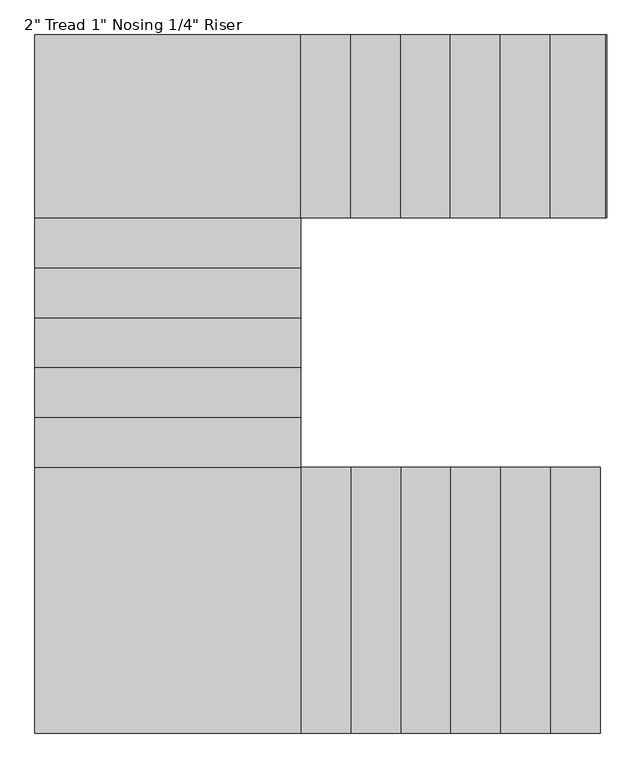
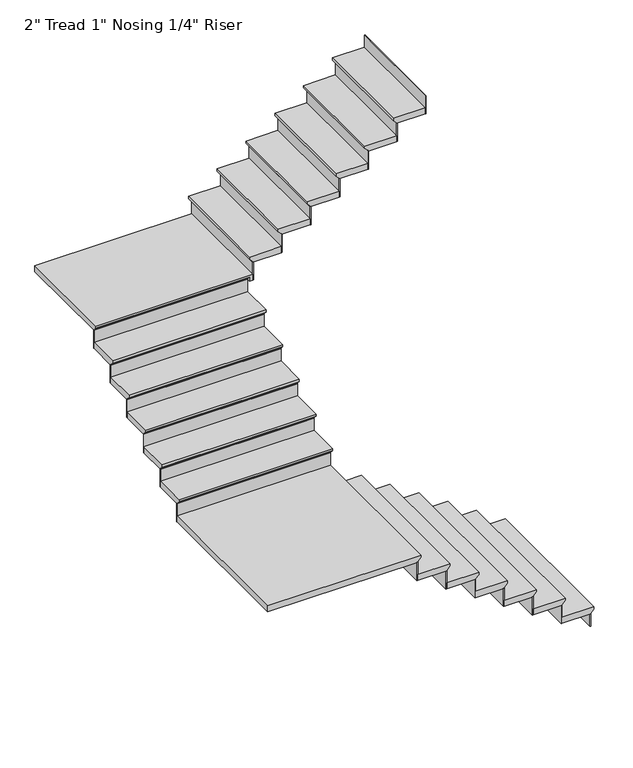
"""IFC4 building model written with IfcOpenShell, lengths in millimetres: stair flight geometry."""

from ifc_helpers import new_model, si_unit, origin, place, context, project, spatial, faceted_brep, source, transform, mapped, element, save


def stair_flight_6293cd8f(model_context):
    return source(origin(), model_context, "Body", "Brep", [
        faceted_brep([(-2515.2117403, -5163.0426559, 133.35), (-2515.2117403, -5163.0426559, 152.4), (-2515.2117403, -6382.2426559, 152.4), (-2515.2117403, -6382.2426559, 133.35), (-2540.6117403, -5163.0426559, 107.95), (-2540.6117403, -6382.2426559, 107.95), (-2769.2117403, -5163.0426559, 152.4), (-2769.2117403, -6382.2426559, 152.4), (-2540.6117403, -6382.2426559, 101.6), (-2769.2117403, -6382.2426559, 101.6), (-2769.2117403, -5163.0426559, 101.6), (-2540.6117403, -5163.0426559, 101.6)], [[[0, 1, 2, 3]], [[4, 0, 3, 5]], [[2, 1, 6, 7]], [[8, 9, 10, 11]], [[2, 7, 9, 8, 5, 3]], [[8, 11, 4, 5]], [[6, 1, 0, 4, 11, 10]], [[7, 6, 10, 9]]]),
        faceted_brep([(-2540.6117403, -5163.0426559, 101.6), (-2540.6117403, -5163.0426559, 0.0), (-2546.9617403, -5163.0426559, 0.0), (-2546.9617403, -5163.0426559, 101.6), (-2540.6117403, -6382.2426559, 101.6), (-2546.9617403, -6382.2426559, 101.6), (-2546.9617403, -6382.2426559, 0.0), (-2540.6117403, -6382.2426559, 0.0)], [[[0, 1, 2, 3]], [[4, 5, 6, 7]], [[1, 0, 4, 7]], [[2, 1, 7, 6]], [[3, 2, 6, 5]], [[0, 3, 5, 4]]]),
        faceted_brep([(-2769.2117403, -5163.0426559, 254.0), (-2769.2117403, -5163.0426559, 101.6), (-2775.5617403, -5163.0426559, 101.6), (-2775.5617403, -5163.0426559, 254.0), (-2769.2117403, -6382.2426559, 254.0), (-2775.5617403, -6382.2426559, 254.0), (-2775.5617403, -6382.2426559, 101.6), (-2769.2117403, -6382.2426559, 101.6)], [[[0, 1, 2, 3]], [[4, 5, 6, 7]], [[1, 0, 4, 7]], [[2, 1, 7, 6]], [[3, 2, 6, 5]], [[0, 3, 5, 4]]]),
        faceted_brep([(-2743.8117403, -6382.2426559, 304.8), (-2743.8117403, -5163.0426559, 304.8), (-2997.8117403, -5163.0426559, 304.8), (-2997.8117403, -6382.2426559, 304.8), (-2769.2117403, -6382.2426559, 254.0), (-2997.8117403, -6382.2426559, 254.0), (-2997.8117403, -5163.0426559, 254.0), (-2769.2117403, -5163.0426559, 254.0), (-2769.2117403, -6382.2426559, 260.35), (-2743.8117403, -6382.2426559, 285.75), (-2769.2117403, -5163.0426559, 260.35), (-2743.8117403, -5163.0426559, 285.75)], [[[0, 1, 2, 3]], [[4, 5, 6, 7]], [[0, 3, 5, 4, 8, 9]], [[4, 7, 10, 8]], [[2, 1, 11, 10, 7, 6]], [[3, 2, 6, 5]], [[11, 1, 0, 9]], [[10, 11, 9, 8]]]),
        faceted_brep([(-2997.8117403, -5163.0426559, 406.4), (-2997.8117403, -5163.0426559, 254.0), (-3004.1617403, -5163.0426559, 254.0), (-3004.1617403, -5163.0426559, 406.4), (-2997.8117403, -6382.2426559, 406.4), (-3004.1617403, -6382.2426559, 406.4), (-3004.1617403, -6382.2426559, 254.0), (-2997.8117403, -6382.2426559, 254.0)], [[[0, 1, 2, 3]], [[4, 5, 6, 7]], [[1, 0, 4, 7]], [[2, 1, 7, 6]], [[3, 2, 6, 5]], [[0, 3, 5, 4]]]),
        faceted_brep([(-2972.4117403, -6382.2426559, 457.2), (-2972.4117403, -5163.0426559, 457.2), (-3226.4117403, -5163.0426559, 457.2), (-3226.4117403, -6382.2426559, 457.2), (-2997.8117403, -6382.2426559, 406.4), (-3226.4117403, -6382.2426559, 406.4), (-3226.4117403, -5163.0426559, 406.4), (-2997.8117403, -5163.0426559, 406.4), (-2997.8117403, -6382.2426559, 412.75), (-2972.4117403, -6382.2426559, 438.15), (-2997.8117403, -5163.0426559, 412.75), (-2972.4117403, -5163.0426559, 438.15)], [[[0, 1, 2, 3]], [[4, 5, 6, 7]], [[0, 3, 5, 4, 8, 9]], [[4, 7, 10, 8]], [[2, 1, 11, 10, 7, 6]], [[3, 2, 6, 5]], [[11, 1, 0, 9]], [[10, 11, 9, 8]]]),
        faceted_brep([(-3226.4117403, -5163.0426559, 558.8), (-3226.4117403, -5163.0426559, 406.4), (-3232.7617403, -5163.0426559, 406.4), (-3232.7617403, -5163.0426559, 558.8), (-3226.4117403, -6382.2426559, 558.8), (-3232.7617403, -6382.2426559, 558.8), (-3232.7617403, -6382.2426559, 406.4), (-3226.4117403, -6382.2426559, 406.4)], [[[0, 1, 2, 3]], [[4, 5, 6, 7]], [[1, 0, 4, 7]], [[2, 1, 7, 6]], [[3, 2, 6, 5]], [[0, 3, 5, 4]]]),
        faceted_brep([(-3201.0117403, -6382.2426559, 609.6), (-3201.0117403, -5163.0426559, 609.6), (-3455.0117403, -5163.0426559, 609.6), (-3455.0117403, -6382.2426559, 609.6), (-3226.4117403, -6382.2426559, 558.8), (-3455.0117403, -6382.2426559, 558.8), (-3455.0117403, -5163.0426559, 558.8), (-3226.4117403, -5163.0426559, 558.8), (-3226.4117403, -6382.2426559, 565.15), (-3201.0117403, -6382.2426559, 590.55), (-3226.4117403, -5163.0426559, 565.15), (-3201.0117403, -5163.0426559, 590.55)], [[[0, 1, 2, 3]], [[4, 5, 6, 7]], [[0, 3, 5, 4, 8, 9]], [[4, 7, 10, 8]], [[2, 1, 11, 10, 7, 6]], [[3, 2, 6, 5]], [[11, 1, 0, 9]], [[10, 11, 9, 8]]]),
        faceted_brep([(-3455.0117403, -5163.0426559, 711.2), (-3455.0117403, -5163.0426559, 558.8), (-3461.3617403, -5163.0426559, 558.8), (-3461.3617403, -5163.0426559, 711.2), (-3455.0117403, -6382.2426559, 711.2), (-3461.3617403, -6382.2426559, 711.2), (-3461.3617403, -6382.2426559, 558.8), (-3455.0117403, -6382.2426559, 558.8)], [[[0, 1, 2, 3]], [[4, 5, 6, 7]], [[1, 0, 4, 7]], [[2, 1, 7, 6]], [[3, 2, 6, 5]], [[0, 3, 5, 4]]]),
        faceted_brep([(-3429.6117403, -6382.2426559, 762.0), (-3429.6117403, -5163.0426559, 762.0), (-3683.6117403, -5163.0426559, 762.0), (-3683.6117403, -6382.2426559, 762.0), (-3455.0117403, -6382.2426559, 711.2), (-3683.6117403, -6382.2426559, 711.2), (-3683.6117403, -5163.0426559, 711.2), (-3455.0117403, -5163.0426559, 711.2), (-3455.0117403, -6382.2426559, 717.55), (-3429.6117403, -6382.2426559, 742.95), (-3455.0117403, -5163.0426559, 717.55), (-3429.6117403, -5163.0426559, 742.95)], [[[0, 1, 2, 3]], [[4, 5, 6, 7]], [[0, 3, 5, 4, 8, 9]], [[4, 7, 10, 8]], [[2, 1, 11, 10, 7, 6]], [[3, 2, 6, 5]], [[11, 1, 0, 9]], [[10, 11, 9, 8]]]),
        faceted_brep([(-3683.6117403, -5163.0426559, 863.6), (-3683.6117403, -5163.0426559, 711.2), (-3689.9617403, -5163.0426559, 711.2), (-3689.9617403, -5163.0426559, 863.6), (-3683.6117403, -6382.2426559, 863.6), (-3689.9617403, -6382.2426559, 863.6), (-3689.9617403, -6382.2426559, 711.2), (-3683.6117403, -6382.2426559, 711.2)], [[[0, 1, 2, 3]], [[4, 5, 6, 7]], [[1, 0, 4, 7]], [[2, 1, 7, 6]], [[3, 2, 6, 5]], [[0, 3, 5, 4]]]),
        faceted_brep([(-3658.2117403, -6382.2426559, 914.4), (-3658.2117403, -5163.0426559, 914.4), (-3912.2117403, -5163.0426559, 914.4), (-3912.2117403, -6382.2426559, 914.4), (-3683.6117403, -6382.2426559, 863.6), (-3912.2117403, -6382.2426559, 863.6), (-3912.2117403, -5163.0426559, 863.6), (-3683.6117403, -5163.0426559, 863.6), (-3683.6117403, -6382.2426559, 869.95), (-3658.2117403, -6382.2426559, 895.35), (-3683.6117403, -5163.0426559, 869.95), (-3658.2117403, -5163.0426559, 895.35)], [[[0, 1, 2, 3]], [[4, 5, 6, 7]], [[0, 3, 5, 4, 8, 9]], [[4, 7, 10, 8]], [[2, 1, 11, 10, 7, 6]], [[3, 2, 6, 5]], [[11, 1, 0, 9]], [[10, 11, 9, 8]]]),
        faceted_brep([(-3912.2117403, -5163.0426559, 1016.0), (-3912.2117403, -5163.0426559, 863.6), (-3918.5617403, -5163.0426559, 863.6), (-3918.5617403, -5163.0426559, 1016.0), (-3912.2117403, -6382.2426559, 1016.0), (-3918.5617403, -6382.2426559, 1016.0), (-3918.5617403, -6382.2426559, 863.6), (-3912.2117403, -6382.2426559, 863.6)], [[[0, 1, 2, 3]], [[4, 5, 6, 7]], [[1, 0, 4, 7]], [[2, 1, 7, 6]], [[3, 2, 6, 5]], [[0, 3, 5, 4]]]),
        faceted_brep([(-5106.0117403, -5137.6426559, 1066.8), (-5106.0117403, -6382.2426559, 1066.8), (-3886.8117403, -6382.2426559, 1066.8), (-3886.8117403, -5137.6426559, 1066.8), (-5106.0117403, -6382.2426559, 1016.0), (-5106.0117403, -5137.6426559, 1016.0), (-3886.8117403, -5137.6426559, 1016.0), (-3886.8117403, -5163.0426559, 1016.0), (-3912.2117403, -5163.0426559, 1016.0), (-3912.2117403, -6382.2426559, 1016.0), (-3912.2117403, -6382.2426559, 1022.35), (-3886.8117403, -6382.2426559, 1047.75), (-3912.2117403, -5163.0426559, 1022.35), (-3886.8117403, -5163.0426559, 1047.75)], [[[0, 1, 2, 3]], [[4, 5, 6, 7, 8, 9]], [[1, 0, 5, 4]], [[2, 1, 4, 9, 10, 11]], [[9, 8, 12, 10]], [[8, 7, 13, 12]], [[3, 2, 11, 13, 7, 6]], [[0, 3, 6, 5]], [[11, 10, 12, 13]]]),
        faceted_brep([(-3886.8117403, -5137.6426559, 1168.4), (-3886.8117403, -5137.6426559, 1016.0), (-3886.8117403, -5131.2926559, 1016.0), (-3886.8117403, -5131.2926559, 1168.4), (-5106.0117403, -5137.6426559, 1168.4), (-5106.0117403, -5131.2926559, 1168.4), (-5106.0117403, -5131.2926559, 1016.0), (-5106.0117403, -5137.6426559, 1016.0)], [[[0, 1, 2, 3]], [[4, 5, 6, 7]], [[1, 0, 4, 7]], [[2, 1, 7, 6]], [[3, 2, 6, 5]], [[0, 3, 5, 4]]]),
        faceted_brep([(-5106.0117403, -5163.0426559, 1219.2), (-3886.8117403, -5163.0426559, 1219.2), (-3886.8117403, -4909.0426559, 1219.2), (-5106.0117403, -4909.0426559, 1219.2), (-5106.0117403, -5137.6426559, 1168.4), (-5106.0117403, -4909.0426559, 1168.4), (-3886.8117403, -4909.0426559, 1168.4), (-3886.8117403, -5137.6426559, 1168.4), (-5106.0117403, -5137.6426559, 1174.75), (-5106.0117403, -5163.0426559, 1200.15), (-3886.8117403, -5137.6426559, 1174.75), (-3886.8117403, -5163.0426559, 1200.15)], [[[0, 1, 2, 3]], [[4, 5, 6, 7]], [[0, 3, 5, 4, 8, 9]], [[4, 7, 10, 8]], [[2, 1, 11, 10, 7, 6]], [[3, 2, 6, 5]], [[11, 1, 0, 9]], [[10, 11, 9, 8]]]),
        faceted_brep([(-3886.8117403, -4909.0426559, 1320.8), (-3886.8117403, -4909.0426559, 1168.4), (-3886.8117403, -4902.6926559, 1168.4), (-3886.8117403, -4902.6926559, 1320.8), (-5106.0117403, -4909.0426559, 1320.8), (-5106.0117403, -4902.6926559, 1320.8), (-5106.0117403, -4902.6926559, 1168.4), (-5106.0117403, -4909.0426559, 1168.4)], [[[0, 1, 2, 3]], [[4, 5, 6, 7]], [[1, 0, 4, 7]], [[2, 1, 7, 6]], [[3, 2, 6, 5]], [[0, 3, 5, 4]]]),
        faceted_brep([(-5106.0117403, -4934.4426559, 1371.6), (-3886.8117403, -4934.4426559, 1371.6), (-3886.8117403, -4680.4426559, 1371.6), (-5106.0117403, -4680.4426559, 1371.6), (-5106.0117403, -4909.0426559, 1320.8), (-5106.0117403, -4680.4426559, 1320.8), (-3886.8117403, -4680.4426559, 1320.8), (-3886.8117403, -4909.0426559, 1320.8), (-5106.0117403, -4909.0426559, 1327.15), (-5106.0117403, -4934.4426559, 1352.55), (-3886.8117403, -4909.0426559, 1327.15), (-3886.8117403, -4934.4426559, 1352.55)], [[[0, 1, 2, 3]], [[4, 5, 6, 7]], [[0, 3, 5, 4, 8, 9]], [[4, 7, 10, 8]], [[2, 1, 11, 10, 7, 6]], [[3, 2, 6, 5]], [[11, 1, 0, 9]], [[10, 11, 9, 8]]]),
        faceted_brep([(-3886.8117403, -4680.4426559, 1473.2), (-3886.8117403, -4680.4426559, 1320.8), (-3886.8117403, -4674.0926559, 1320.8), (-3886.8117403, -4674.0926559, 1473.2), (-5106.0117403, -4680.4426559, 1473.2), (-5106.0117403, -4674.0926559, 1473.2), (-5106.0117403, -4674.0926559, 1320.8), (-5106.0117403, -4680.4426559, 1320.8)], [[[0, 1, 2, 3]], [[4, 5, 6, 7]], [[1, 0, 4, 7]], [[2, 1, 7, 6]], [[3, 2, 6, 5]], [[0, 3, 5, 4]]]),
        faceted_brep([(-5106.0117403, -4705.8426559, 1524.0), (-3886.8117403, -4705.8426559, 1524.0), (-3886.8117403, -4451.8426559, 1524.0), (-5106.0117403, -4451.8426559, 1524.0), (-5106.0117403, -4680.4426559, 1473.2), (-5106.0117403, -4451.8426559, 1473.2), (-3886.8117403, -4451.8426559, 1473.2), (-3886.8117403, -4680.4426559, 1473.2), (-5106.0117403, -4680.4426559, 1479.55), (-5106.0117403, -4705.8426559, 1504.95), (-3886.8117403, -4680.4426559, 1479.55), (-3886.8117403, -4705.8426559, 1504.95)], [[[0, 1, 2, 3]], [[4, 5, 6, 7]], [[0, 3, 5, 4, 8, 9]], [[4, 7, 10, 8]], [[2, 1, 11, 10, 7, 6]], [[3, 2, 6, 5]], [[11, 1, 0, 9]], [[10, 11, 9, 8]]]),
        faceted_brep([(-3886.8117403, -4451.8426559, 1625.6), (-3886.8117403, -4451.8426559, 1473.2), (-3886.8117403, -4445.4926559, 1473.2), (-3886.8117403, -4445.4926559, 1625.6), (-5106.0117403, -4451.8426559, 1625.6), (-5106.0117403, -4445.4926559, 1625.6), (-5106.0117403, -4445.4926559, 1473.2), (-5106.0117403, -4451.8426559, 1473.2)], [[[0, 1, 2, 3]], [[4, 5, 6, 7]], [[1, 0, 4, 7]], [[2, 1, 7, 6]], [[3, 2, 6, 5]], [[0, 3, 5, 4]]]),
        faceted_brep([(-5106.0117403, -4477.2426559, 1676.4), (-3886.8117403, -4477.2426559, 1676.4), (-3886.8117403, -4223.2426559, 1676.4), (-5106.0117403, -4223.2426559, 1676.4), (-5106.0117403, -4451.8426559, 1625.6), (-5106.0117403, -4223.2426559, 1625.6), (-3886.8117403, -4223.2426559, 1625.6), (-3886.8117403, -4451.8426559, 1625.6), (-5106.0117403, -4451.8426559, 1631.95), (-5106.0117403, -4477.2426559, 1657.35), (-3886.8117403, -4451.8426559, 1631.95), (-3886.8117403, -4477.2426559, 1657.35)], [[[0, 1, 2, 3]], [[4, 5, 6, 7]], [[0, 3, 5, 4, 8, 9]], [[4, 7, 10, 8]], [[2, 1, 11, 10, 7, 6]], [[3, 2, 6, 5]], [[11, 1, 0, 9]], [[10, 11, 9, 8]]]),
        faceted_brep([(-3886.8117403, -4223.2426559, 1778.0), (-3886.8117403, -4223.2426559, 1625.6), (-3886.8117403, -4216.8926559, 1625.6), (-3886.8117403, -4216.8926559, 1778.0), (-5106.0117403, -4223.2426559, 1778.0), (-5106.0117403, -4216.8926559, 1778.0), (-5106.0117403, -4216.8926559, 1625.6), (-5106.0117403, -4223.2426559, 1625.6)], [[[0, 1, 2, 3]], [[4, 5, 6, 7]], [[1, 0, 4, 7]], [[2, 1, 7, 6]], [[3, 2, 6, 5]], [[0, 3, 5, 4]]]),
        faceted_brep([(-5106.0117403, -4248.6426559, 1828.8), (-3886.8117403, -4248.6426559, 1828.8), (-3886.8117403, -3994.6426559, 1828.8), (-5106.0117403, -3994.6426559, 1828.8), (-5106.0117403, -4223.2426559, 1778.0), (-5106.0117403, -3994.6426559, 1778.0), (-3886.8117403, -3994.6426559, 1778.0), (-3886.8117403, -4223.2426559, 1778.0), (-5106.0117403, -4223.2426559, 1784.35), (-5106.0117403, -4248.6426559, 1809.75), (-3886.8117403, -4223.2426559, 1784.35), (-3886.8117403, -4248.6426559, 1809.75)], [[[0, 1, 2, 3]], [[4, 5, 6, 7]], [[0, 3, 5, 4, 8, 9]], [[4, 7, 10, 8]], [[2, 1, 11, 10, 7, 6]], [[3, 2, 6, 5]], [[11, 1, 0, 9]], [[10, 11, 9, 8]]]),
        faceted_brep([(-3886.8117403, -3994.6426559, 1930.4), (-3886.8117403, -3994.6426559, 1778.0), (-3886.8117403, -3988.2926559, 1778.0), (-3886.8117403, -3988.2926559, 1930.4), (-5106.0117403, -3994.6426559, 1930.4), (-5106.0117403, -3988.2926559, 1930.4), (-5106.0117403, -3988.2926559, 1778.0), (-5106.0117403, -3994.6426559, 1778.0)], [[[0, 1, 2, 3]], [[4, 5, 6, 7]], [[1, 0, 4, 7]], [[2, 1, 7, 6]], [[3, 2, 6, 5]], [[0, 3, 5, 4]]]),
        faceted_brep([(-3861.4117403, -3181.8426559, 1981.2), (-5106.0117403, -3181.8426559, 1981.2), (-5106.0117403, -4020.0426559, 1981.2), (-3861.4117403, -4020.0426559, 1981.2), (-5106.0117403, -3181.8426559, 1930.4), (-3861.4117403, -3181.8426559, 1930.4), (-3861.4117403, -4020.0426559, 1930.4), (-3886.8117403, -4020.0426559, 1930.4), (-3886.8117403, -3994.6426559, 1930.4), (-5106.0117403, -3994.6426559, 1930.4), (-5106.0117403, -3994.6426559, 1936.75), (-5106.0117403, -4020.0426559, 1962.15), (-3886.8117403, -3994.6426559, 1936.75), (-3886.8117403, -4020.0426559, 1962.15)], [[[0, 1, 2, 3]], [[4, 5, 6, 7, 8, 9]], [[1, 0, 5, 4]], [[2, 1, 4, 9, 10, 11]], [[9, 8, 12, 10]], [[8, 7, 13, 12]], [[3, 2, 11, 13, 7, 6]], [[0, 3, 6, 5]], [[11, 10, 12, 13]]]),
        faceted_brep([(-3861.4117403, -4020.0426559, 2082.8), (-3861.4117403, -4020.0426559, 1930.4), (-3855.0617403, -4020.0426559, 1930.4), (-3855.0617403, -4020.0426559, 2082.8), (-3861.4117403, -3181.8426559, 2082.8), (-3855.0617403, -3181.8426559, 2082.8), (-3855.0617403, -3181.8426559, 1930.4), (-3861.4117403, -3181.8426559, 1930.4)], [[[0, 1, 2, 3]], [[4, 5, 6, 7]], [[1, 0, 4, 7]], [[2, 1, 7, 6]], [[3, 2, 6, 5]], [[0, 3, 5, 4]]]),
        faceted_brep([(-3886.8117403, -3181.8426559, 2133.6), (-3886.8117403, -4020.0426559, 2133.6), (-3632.8117403, -4020.0426559, 2133.6), (-3632.8117403, -3181.8426559, 2133.6), (-3861.4117403, -3181.8426559, 2082.8), (-3632.8117403, -3181.8426559, 2082.8), (-3632.8117403, -4020.0426559, 2082.8), (-3861.4117403, -4020.0426559, 2082.8), (-3861.4117403, -3181.8426559, 2089.15), (-3886.8117403, -3181.8426559, 2114.55), (-3861.4117403, -4020.0426559, 2089.15), (-3886.8117403, -4020.0426559, 2114.55)], [[[0, 1, 2, 3]], [[4, 5, 6, 7]], [[0, 3, 5, 4, 8, 9]], [[4, 7, 10, 8]], [[2, 1, 11, 10, 7, 6]], [[3, 2, 6, 5]], [[11, 1, 0, 9]], [[10, 11, 9, 8]]]),
        faceted_brep([(-3632.8117403, -4020.0426559, 2235.2), (-3632.8117403, -4020.0426559, 2082.8), (-3626.4617403, -4020.0426559, 2082.8), (-3626.4617403, -4020.0426559, 2235.2), (-3632.8117403, -3181.8426559, 2235.2), (-3626.4617403, -3181.8426559, 2235.2), (-3626.4617403, -3181.8426559, 2082.8), (-3632.8117403, -3181.8426559, 2082.8)], [[[0, 1, 2, 3]], [[4, 5, 6, 7]], [[1, 0, 4, 7]], [[2, 1, 7, 6]], [[3, 2, 6, 5]], [[0, 3, 5, 4]]]),
        faceted_brep([(-3658.2117403, -3181.8426559, 2286.0), (-3658.2117403, -4020.0426559, 2286.0), (-3404.2117403, -4020.0426559, 2286.0), (-3404.2117403, -3181.8426559, 2286.0), (-3632.8117403, -3181.8426559, 2235.2), (-3404.2117403, -3181.8426559, 2235.2), (-3404.2117403, -4020.0426559, 2235.2), (-3632.8117403, -4020.0426559, 2235.2), (-3632.8117403, -3181.8426559, 2241.55), (-3658.2117403, -3181.8426559, 2266.95), (-3632.8117403, -4020.0426559, 2241.55), (-3658.2117403, -4020.0426559, 2266.95)], [[[0, 1, 2, 3]], [[4, 5, 6, 7]], [[0, 3, 5, 4, 8, 9]], [[4, 7, 10, 8]], [[2, 1, 11, 10, 7, 6]], [[3, 2, 6, 5]], [[11, 1, 0, 9]], [[10, 11, 9, 8]]]),
        faceted_brep([(-3404.2117403, -4020.0426559, 2387.6), (-3404.2117403, -4020.0426559, 2235.2), (-3397.8617403, -4020.0426559, 2235.2), (-3397.8617403, -4020.0426559, 2387.6), (-3404.2117403, -3181.8426559, 2387.6), (-3397.8617403, -3181.8426559, 2387.6), (-3397.8617403, -3181.8426559, 2235.2), (-3404.2117403, -3181.8426559, 2235.2)], [[[0, 1, 2, 3]], [[4, 5, 6, 7]], [[1, 0, 4, 7]], [[2, 1, 7, 6]], [[3, 2, 6, 5]], [[0, 3, 5, 4]]]),
        faceted_brep([(-3429.6117403, -3181.8426559, 2438.4), (-3429.6117403, -4020.0426559, 2438.4), (-3175.6117403, -4020.0426559, 2438.4), (-3175.6117403, -3181.8426559, 2438.4), (-3404.2117403, -3181.8426559, 2387.6), (-3175.6117403, -3181.8426559, 2387.6), (-3175.6117403, -4020.0426559, 2387.6), (-3404.2117403, -4020.0426559, 2387.6), (-3404.2117403, -3181.8426559, 2393.95), (-3429.6117403, -3181.8426559, 2419.35), (-3404.2117403, -4020.0426559, 2393.95), (-3429.6117403, -4020.0426559, 2419.35)], [[[0, 1, 2, 3]], [[4, 5, 6, 7]], [[0, 3, 5, 4, 8, 9]], [[4, 7, 10, 8]], [[2, 1, 11, 10, 7, 6]], [[3, 2, 6, 5]], [[11, 1, 0, 9]], [[10, 11, 9, 8]]]),
        faceted_brep([(-3175.6117403, -4020.0426559, 2540.0), (-3175.6117403, -4020.0426559, 2387.6), (-3169.2617403, -4020.0426559, 2387.6), (-3169.2617403, -4020.0426559, 2540.0), (-3175.6117403, -3181.8426559, 2540.0), (-3169.2617403, -3181.8426559, 2540.0), (-3169.2617403, -3181.8426559, 2387.6), (-3175.6117403, -3181.8426559, 2387.6)], [[[0, 1, 2, 3]], [[4, 5, 6, 7]], [[1, 0, 4, 7]], [[2, 1, 7, 6]], [[3, 2, 6, 5]], [[0, 3, 5, 4]]]),
        faceted_brep([(-3201.0117403, -3181.8426559, 2590.8), (-3201.0117403, -4020.0426559, 2590.8), (-2947.0117403, -4020.0426559, 2590.8), (-2947.0117403, -3181.8426559, 2590.8), (-3175.6117403, -3181.8426559, 2540.0), (-2947.0117403, -3181.8426559, 2540.0), (-2947.0117403, -4020.0426559, 2540.0), (-3175.6117403, -4020.0426559, 2540.0), (-3175.6117403, -3181.8426559, 2546.35), (-3201.0117403, -3181.8426559, 2571.75), (-3175.6117403, -4020.0426559, 2546.35), (-3201.0117403, -4020.0426559, 2571.75)], [[[0, 1, 2, 3]], [[4, 5, 6, 7]], [[0, 3, 5, 4, 8, 9]], [[4, 7, 10, 8]], [[2, 1, 11, 10, 7, 6]], [[3, 2, 6, 5]], [[11, 1, 0, 9]], [[10, 11, 9, 8]]]),
        faceted_brep([(-2947.0117403, -4020.0426559, 2692.4), (-2947.0117403, -4020.0426559, 2540.0), (-2940.6617403, -4020.0426559, 2540.0), (-2940.6617403, -4020.0426559, 2692.4), (-2947.0117403, -3181.8426559, 2692.4), (-2940.6617403, -3181.8426559, 2692.4), (-2940.6617403, -3181.8426559, 2540.0), (-2947.0117403, -3181.8426559, 2540.0)], [[[0, 1, 2, 3]], [[4, 5, 6, 7]], [[1, 0, 4, 7]], [[2, 1, 7, 6]], [[3, 2, 6, 5]], [[0, 3, 5, 4]]]),
        faceted_brep([(-2972.4117403, -3181.8426559, 2743.2), (-2972.4117403, -4020.0426559, 2743.2), (-2718.4117403, -4020.0426559, 2743.2), (-2718.4117403, -3181.8426559, 2743.2), (-2947.0117403, -3181.8426559, 2692.4), (-2718.4117403, -3181.8426559, 2692.4), (-2718.4117403, -4020.0426559, 2692.4), (-2947.0117403, -4020.0426559, 2692.4), (-2947.0117403, -3181.8426559, 2698.75), (-2972.4117403, -3181.8426559, 2724.15), (-2947.0117403, -4020.0426559, 2698.75), (-2972.4117403, -4020.0426559, 2724.15)], [[[0, 1, 2, 3]], [[4, 5, 6, 7]], [[0, 3, 5, 4, 8, 9]], [[4, 7, 10, 8]], [[2, 1, 11, 10, 7, 6]], [[3, 2, 6, 5]], [[11, 1, 0, 9]], [[10, 11, 9, 8]]]),
        faceted_brep([(-2718.4117403, -4020.0426559, 2844.8), (-2718.4117403, -4020.0426559, 2692.4), (-2712.0617403, -4020.0426559, 2692.4), (-2712.0617403, -4020.0426559, 2844.8), (-2718.4117403, -3181.8426559, 2844.8), (-2712.0617403, -3181.8426559, 2844.8), (-2712.0617403, -3181.8426559, 2692.4), (-2718.4117403, -3181.8426559, 2692.4)], [[[0, 1, 2, 3]], [[4, 5, 6, 7]], [[1, 0, 4, 7]], [[2, 1, 7, 6]], [[3, 2, 6, 5]], [[0, 3, 5, 4]]]),
        faceted_brep([(-2489.8117403, -4020.0426559, 2997.2), (-2489.8117403, -4020.0426559, 2844.8), (-2483.4617403, -4020.0426559, 2844.8), (-2483.4617403, -4020.0426559, 2997.2), (-2489.8117403, -3181.8426559, 2997.2), (-2483.4617403, -3181.8426559, 2997.2), (-2483.4617403, -3181.8426559, 2844.8), (-2489.8117403, -3181.8426559, 2844.8)], [[[0, 1, 2, 3]], [[4, 5, 6, 7]], [[1, 0, 4, 7]], [[2, 1, 7, 6]], [[3, 2, 6, 5]], [[0, 3, 5, 4]]]),
        faceted_brep([(-2743.8117403, -3181.8426559, 2895.6), (-2743.8117403, -4020.0426559, 2895.6), (-2489.8117403, -4020.0426559, 2895.6), (-2489.8117403, -3181.8426559, 2895.6), (-2718.4117403, -3181.8426559, 2844.8), (-2489.8117403, -3181.8426559, 2844.8), (-2489.8117403, -4020.0426559, 2844.8), (-2718.4117403, -4020.0426559, 2844.8), (-2718.4117403, -3181.8426559, 2851.15), (-2743.8117403, -3181.8426559, 2876.55), (-2718.4117403, -4020.0426559, 2851.15), (-2743.8117403, -4020.0426559, 2876.55)], [[[0, 1, 2, 3]], [[4, 5, 6, 7]], [[0, 3, 5, 4, 8, 9]], [[4, 7, 10, 8]], [[2, 1, 11, 10, 7, 6]], [[3, 2, 6, 5]], [[11, 1, 0, 9]], [[10, 11, 9, 8]]]),
    ])


if __name__ == "__main__":
    model = new_model("IFC4")
    model_context = context("Model", 3, world=origin())
    ifc_project = project(units=[si_unit("LENGTHUNIT", "METRE", prefix="MILLI")], contexts=[model_context])
    site = spatial("IfcSite", under=ifc_project)
    building = spatial("IfcBuilding", under=site)
    placement = place(None, origin())
    stair_flight_shape = stair_flight_6293cd8f(model_context)
    element("IfcStairFlight", 1, ObjectType="2\" Tread 1\" Nosing 1/4\" Riser", at=placement, inside=building, context=model_context, shape_type="MappedRepresentation", body=[
        mapped(stair_flight_shape, transform((0.0, 0.0, 0.0), x_axis=(1.0, 0.0, 0.0), y_axis=(0.0, 1.0, 0.0), z_axis=(0.0, 0.0, 1.0))),
    ])
    save(model, "model.ifc")

# Revit data of these elements
# Element 1 (IfcStairFlight, "2\" Tread 1\" Nosing 1/4\" Riser")
#   Materials on its faces: "Wood Planks"
# Materials
#   "Wood Planks": class "Wood", colour RGB 193 160 115, transparency 0, Description = "Physical material.", Cost = 0
